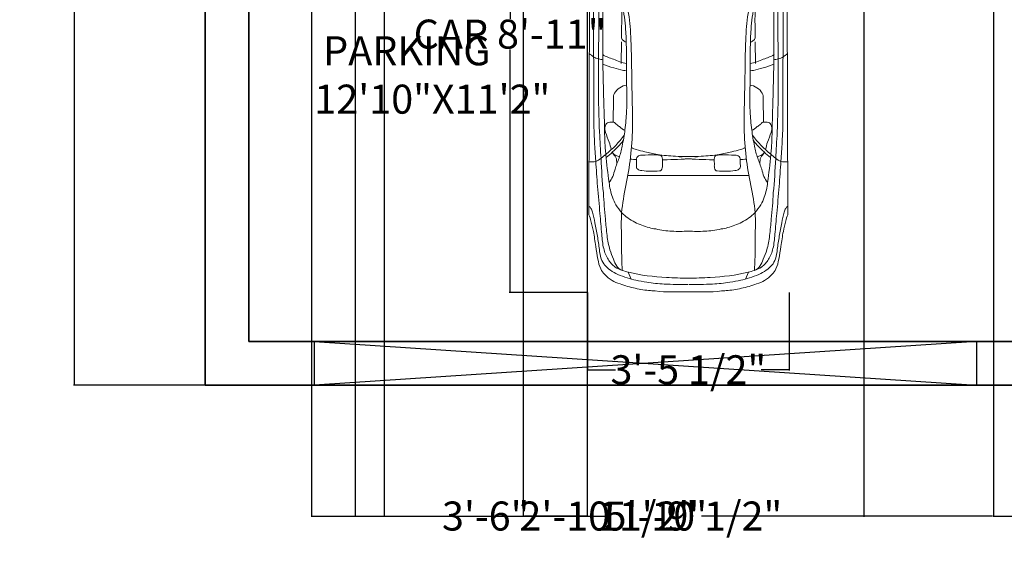
# Model space of a CAD drawing. Units: inches. Extents: x 3398 to 3816, y 15195 to 15771.
# Tile 1 of 10: x 3405 to 3608, y 15195 to 15306. Entities that reach past the tile are written whole.
import ezdxf

# ---------------------------------------------------------------- set-up
doc = ezdxf.new("R2010")
doc.units = ezdxf.units.IN
doc.header["$MEASUREMENT"] = 0
for name, color, linetype, lineweight in [('A-ANNO-DIMS', 2, 'Continuous', 18), ('A-AREA-IDEN', 7, 'Continuous', 25), ('C-PKNG-VEHI', 8, 'Continuous', 13), ('C-PROP', 7, 'Continuous', 35), ('C-SITE-GATE', 4, 'Continuous', 25)]:
    doc.layers.add(name, color=color, linetype=linetype, lineweight=lineweight)
doc.styles.get("Standard").update_dxf_attribs({"font": 'arial.ttf'})
doc.dimstyles.get("Standard").update_dxf_attribs({"dimtxt": 6, "dimasz": 0.18, "dimexe": 0.18, "dimexo": 0.0625, "dimgap": 0.09, "dimtad": 0, "dimtih": 1, "dimtoh": 1, "dimdec": 1, "dimzin": 0, "dimdsep": 46, "dimlunit": 3, "dimtxsty": 'Standard', "dimcen": 0.09, "dimadec": 0, "dimazin": 0, "dimtfac": 1, "dimtdec": 1, "dimtofl": 0, "dimtmove": 0, "dimatfit": 3, "dimfxl": 1, "dimtolj": 1, "dimtzin": 0, "dimarcsym": 0})

# ---------------------------------------------------------------- blocks, each defined once
blk = doc.blocks.new('A$C242571DA')
for p, q in [((1659.9, 1632), (1714.3, 1732.5)), ((1714.3, 1732.5), (3817.1, 1739.9)), ((1638.3, 1618.5), (1625.1, 1632)), ((1625.1, 1632), (1659.9, 1632)), ((1681.8, 1651.6), (2695.2, 1655.3)), ((1699.9, 1699.4), (2984.7, 1695.8)), ((1317.4, 1579.7), (1909.8, 1424.9)), ((1638.3, 1618.5), (2503.3, 1618.5)), ((1659.9, 1548.1), (1638.3, 1618.5)), ((2503.3, 1618.5), (2861.6, 1607.5)), ((1644, 1489.1), (1610.4, 1020.2)), ((2311.9, 1454.3), (2500.6, 1456.9)), ((3007.2, 1526.5), (2808.1, 1525.2)), ((3474.6, 1401.1), (3474.6, 843)), ((4315.2, 1398), (4377.3, 1370.5)), ((1626.1, 1006.5), (1632.8, 719.7)), ((3474.6, 345.6), (3474.6, 903.8)), ((1740.2, 584.9), (1649.3, 586.9)), ((1746.1, 420.6), (1649.3, 420.6)), ((4315.2, 348.7), (4377.3, 376.3)), ((1317.4, 167), (1909.8, 321.9)), ((2311.9, 292.5), (2500.6, 289.8)), ((1659.9, 198.7), (1638.3, 128.2)), ((3007.2, 220.3), (2808.1, 221.6)), ((1638.3, 128.2), (1625.1, 114.7)), ((1625.1, 114.7), (1659.9, 114.7)), ((1638.3, 128.2), (2503.3, 128.2)), ((1659.9, 114.7), (1714.3, 14.2)), ((1681.8, 95.1), (2695.2, 91.4)), ((2503.3, 128.2), (2861.6, 139.2)), ((1699.9, 47.3), (2984.7, 51)), ((1714.3, 14.2), (3817.1, 6.9))]:
    blk.add_line(p, q)
for centre in [(1546.4, 1462.5), (1546.4, 284.2)]:
    blk.add_ellipse(centre, major_axis=(0, 42.9), ratio=0.983266, start_param=4.712389, end_param=10.995574)
for points, knots in [([(0, 873.4), (0, 927.8), (15.6, 1088.6), (25.5, 1309.8), (120.7, 1476.4), (189.2, 1569), (273.5, 1623.1), (369.9, 1666.3), (483, 1694.7), (561.3, 1714.9), (604.6, 1715.7)], [0, 0, 0, 0, 0.16039, 0.479033, 0.632967, 0.722015, 0.817474, 0.927562, 1.03733, 1.167094, 1.167094, 1.167094, 1.167094]), ([(604.6, 1715.7), (545.5, 1714.5), (448.5, 1664.6), (320.8, 1610.6), (225.4, 1521.2), (147.3, 1390.5), (121.7, 1275.2), (113.6, 1208.7)], [0, 0, 0, 0, 0.1772572, 0.3124951, 0.4151678, 0.5597243, 0.7575412, 0.7575412, 0.7575412, 0.7575412]), ([(722.7, 1726.6), (720.8, 1714.9), (694.5, 1689.9), (643, 1671.8), (573.6, 1655.4), (508.5, 1647), (455.2, 1634.7), (428.7, 1627.3), (416.9, 1624.1)], [0, 0, 0, 0, 0.034703, 0.0959761, 0.1659336, 0.2471559, 0.2929944, 0.3295918, 0.3295918, 0.3295918, 0.3295918]), ([(604.6, 1715.7), (642.1, 1723.4), (788.5, 1729.2), (1039.3, 1732.2), (1344.5, 1729.9), (1542, 1733.1), (1633.8, 1733.7)], [0, 0, 0, 0, 0.114897, 0.437061, 0.754269, 1.029686, 1.029686, 1.029686, 1.029686]), ([(1043.6, 1729.2), (1048.6, 1717.9), (1080.9, 1704.2), (1138.6, 1687.6), (1237.7, 1685.6), (1394.7, 1691.3), (1521.7, 1692.4), (1601.5, 1692.7)], [0, 0, 0, 0, 0.0364992, 0.0923739, 0.1867837, 0.3273982, 0.5667068, 0.5667068, 0.5667068, 0.5667068]), ([(1356.8, 1732.2), (1357.1, 1712.8), (1360, 1678.8), (1363.9, 1630.5), (1383.3, 1613.5), (1391, 1607.2)], [0, 0, 0, 0, 1.462159, 2.651105, 3.386321, 3.386321, 3.386321, 3.386321]), ([(1714.3, 1732.5), (1707.7, 1737.6), (1683.3, 1753), (1628.7, 1741.2), (1605.6, 1691.5), (1561.7, 1652.4), (1594.1, 1610.3), (1627.9, 1608.3), (1638.3, 1618.5)], [0, 0, 0, 0, 0.024864, 0.0846267, 0.1362471, 0.1900683, 0.2245199, 0.2681841, 0.2681841, 0.2681841, 0.2681841]), ([(2414.7, 1735), (2424.9, 1723.3), (2447.2, 1698.8), (2461.2, 1657.6), (2468.1, 1629), (2468, 1616.1)], [1.808086, 1.808086, 1.808086, 1.808086, 2.918874, 4.131288, 5.10151, 5.10151, 5.10151, 5.10151]), ([(3356.5, 1739.4), (3354.9, 1719.2), (3360.8, 1678.2), (3324, 1631.5), (3255.4, 1544.3), (3187.1, 1476.2), (3125.2, 1432.2)], [0, 0, 0, 0, 0.0597371, 0.1139981, 0.1672498, 0.3938869, 0.3938869, 0.3938869, 0.3938869]), ([(3745.3, 1736.8), (3748.5, 1730.1), (3764.2, 1717.1), (3811.5, 1698.6), (3894.7, 1686.7), (4002.9, 1663.2), (4107.9, 1648.7), (4195.8, 1638.3), (4258.6, 1603.2), (4302.1, 1549.7), (4339.9, 1483.8), (4365.2, 1407.6), (4389.6, 1324.4), (4397.9, 1266.9), (4401.8, 1235.2)], [0, 0, 0, 0, 0.0219205, 0.0572122, 0.1522539, 0.2718866, 0.3894011, 0.4710097, 0.5346344, 0.5986698, 0.6733118, 0.758696, 0.8351341, 0.9293726, 0.9293726, 0.9293726, 0.9293726]), ([(3817.1, 1739.9), (3833.2, 1729.7), (3882.9, 1718.2), (3973.3, 1695.2), (4085.1, 1680.5), (4193.8, 1662.8), (4280.6, 1644.3), (4343.9, 1598.1), (4390, 1540.3), (4427.4, 1448.7), (4457.8, 1336.6), (4475.7, 1233.4), (4478.4, 1175.1), (4479.3, 1161.6)], [0, 0, 0, 0, 0.056668, 0.14946, 0.28161, 0.392935, 0.481686, 0.542967, 0.622845, 0.69797, 0.833643, 0.965665, 1.00577, 1.00577, 1.00577, 1.00577]), ([(310.7, 1637.3), (282.5, 1613.7), (230.1, 1569.9), (148.7, 1486.2), (84.8, 1361.3), (60, 1219), (32.6, 1054.3), (25.1, 944.9), (25.1, 873.4)], [0, 0, 0, 0, 0.1095129, 0.2035347, 0.3452507, 0.5161382, 0.6275464, 0.8383798, 0.8383798, 0.8383798, 0.8383798]), ([(426.8, 1656.7), (428.5, 1646.6), (426.9, 1625), (399.8, 1616.6), (368.1, 1593.9), (328, 1564.6), (271.6, 1523.9), (237, 1451.9), (196.2, 1376.7), (183.8, 1314.9), (170, 1279.6), (157.2, 1254.2), (133.3, 1244.4), (118.6, 1242.9)], [0, 0, 0, 0, 0.0304541, 0.0502818, 0.0786089, 0.1479133, 0.1986294, 0.2831705, 0.3780326, 0.4523267, 0.4667809, 0.4902599, 0.5347198, 0.5347198, 0.5347198, 0.5347198]), ([(323.7, 1557.5), (344.8, 1571.9), (400.4, 1585.1), (516, 1606.8), (680.3, 1625.8), (885.4, 1635.7), (1116.8, 1642.2), (1346.1, 1644.2), (1504.7, 1644.7), (1574, 1645.7)], [0, 0, 0, 0, 0.076148, 0.165903, 0.355672, 0.569871, 0.782325, 1.050047, 1.257936, 1.257936, 1.257936, 1.257936]), ([(1574, 1645.7), (1572.9, 1638), (1574.1, 1622), (1559.9, 1618.7), (1555.2, 1617.8)], [0, 0, 0, 0, 0.02274132, 0.03717479, 0.03717479, 0.03717479, 0.03717479]), ([(2695.2, 1655.3), (2829.9, 1655.3), (3041.2, 1651.4), (3351.3, 1630.7), (3527.5, 1623.2), (3626.6, 1612)], [0, 0, 0, 0, 0.4042759, 0.6333827, 0.9326252, 0.9326252, 0.9326252, 0.9326252]), ([(2984.7, 1695.8), (3051, 1695.6), (3172.1, 1691.3), (3367.4, 1677.6), (3575.2, 1664.3), (3788.2, 1643.6), (3968, 1628.1), (4103.8, 1616.8), (4203.6, 1578.1), (4271.8, 1519.5), (4300.6, 1452.1), (4341.7, 1305.3), (4361.8, 1111.2), (4367.5, 936.8), (4367.5, 873.4)], [0, 0, 0, 0, 0.198873, 0.363323, 0.587433, 0.823543, 1.004622, 1.129816, 1.230113, 1.320655, 1.388577, 1.443334, 1.771447, 1.958652, 1.958652, 1.958652, 1.958652]), ([(1317.4, 1579.7), (1227.8, 1586.1), (1036, 1584.8), (741.2, 1572.5), (486.1, 1553.3), (333.3, 1534.3), (283.3, 1528.5)], [0, 0, 0, 0, 0.269375, 0.574535, 0.885339, 1.036319, 1.036319, 1.036319, 1.036319]), ([(1555.2, 1617.8), (1527.7, 1617.8), (1472.5, 1620.4), (1392.7, 1608.8), (1318.5, 1591), (1249.4, 1545.5), (1201.4, 1466.7), (1142.8, 1385.7), (1104.8, 1240.4), (1076, 1072.3), (1056.4, 932.4), (1056.4, 873.4)], [0, 0, 0, 0, 0.082256, 0.165174, 0.241383, 0.30939, 0.405348, 0.511507, 0.603349, 0.843635, 1.017671, 1.017671, 1.017671, 1.017671]), ([(1317.4, 1579.7), (1296.6, 1555.5), (1247.9, 1494.4), (1177.6, 1350.5), (1124.2, 1137.4), (1105.5, 964.9), (1105.5, 873.4)], [0, 0, 0, 0, 0.0947759, 0.2311242, 0.4700259, 0.7400315, 0.7400315, 0.7400315, 0.7400315]), ([(1372.8, 1563.1), (1357.2, 1545), (1321.6, 1490.1), (1277, 1385.7), (1232.8, 1244.2), (1211.1, 1069.4), (1196.8, 942.4), (1196.8, 873.4)], [0, 0, 0, 0, 0.0708922, 0.1925846, 0.3348457, 0.5072814, 0.7109928, 0.7109928, 0.7109928, 0.7109928]), ([(3535.9, 1563.1), (3520.1, 1550.9), (3484.4, 1526.1), (3408.2, 1510.9), (3323.4, 1473.1), (3207.9, 1445), (3072.6, 1422.2), (2866.9, 1404.6), (2626.4, 1412.9), (2396.7, 1410.8), (2200.9, 1416.9), (2001.3, 1438.2), (1732.1, 1525.9), (1527.9, 1578.9), (1407.5, 1610.7)], [0, 0, 0, 0, 0.05975, 0.126928, 0.230034, 0.336675, 0.482225, 0.641324, 0.954906, 1.203173, 1.330375, 1.542773, 1.802261, 2.175545, 2.175545, 2.175545, 2.175545]), ([(2424, 1618.7), (2441.5, 1589.9), (2464.2, 1518.9), (2495.4, 1450.9), (2501.6, 1411.3)], [0, 0, 0, 0, 0.1000351, 0.2184418, 0.2184418, 0.2184418, 0.2184418]), ([(2507.7, 1618.4), (2521, 1587.7), (2536.6, 1527.1), (2559.6, 1458.5), (2563.3, 1420.6), (2563.8, 1411.4)], [0, 0, 0, 0, 2.528586, 4.711885, 5.408215, 5.408215, 5.408215, 5.408215]), ([(2861.6, 1607.5), (2921.1, 1607.3), (3047.2, 1600.8), (3191.4, 1602), (3356.6, 1584.1), (3498.3, 1570.6), (3623.2, 1549.4), (3664.1, 1533.3)], [0, 0, 0, 0, 0.1783018, 0.3787173, 0.431954, 0.6762374, 0.8077184, 0.8077184, 0.8077184, 0.8077184]), ([(3248.1, 1545.2), (3226.9, 1550.4), (3176.1, 1562.1), (3113.7, 1592.9), (3052.6, 1605.3), (3010.4, 1578.8), (3010.3, 1545.3), (3010.3, 1515.9), (3033.7, 1500.1), (3052.6, 1465.2), (3078.9, 1443.5), (3084, 1424.4)], [0, 0, 0, 0, 0.0655106, 0.1550445, 0.2094604, 0.2438604, 0.287164, 0.3001388, 0.3275984, 0.3616951, 0.4200969, 0.4200969, 0.4200969, 0.4200969]), ([(3319, 1587.1), (3303.3, 1568.1), (3256.9, 1516.7), (3206.7, 1467.3), (3171.4, 1439.5)], [0, 0, 0, 0, 1.868162, 5.271297, 5.271297, 5.271297, 5.271297]), ([(3626.6, 1612), (3702.5, 1609.1), (3826.2, 1596.8), (3991.4, 1583.2), (4111.7, 1562.4), (4212.2, 1522.7), (4290.4, 1488), (4300.7, 1447.5)], [0, 0, 0, 0, 0.2277977, 0.3719478, 0.4996814, 0.5863441, 0.709615, 0.709615, 0.709615, 0.709615]), ([(1909.8, 1424.9), (1933.5, 1418.7), (1995.6, 1407.6), (2094.4, 1385.8), (2211.8, 1377.1), (2419, 1366.9), (2704.7, 1366.5), (3032.7, 1354.2), (3316.2, 1371), (3558.7, 1415.9), (3789.1, 1461.7), (4028.9, 1452.9), (4196.2, 1455.2), (4292.7, 1447.9), (4300.7, 1447.5)], [0, 0, 0, 0, 0.073325, 0.188896, 0.303039, 0.425821, 0.811242, 1.159737, 1.41058, 1.660623, 1.899627, 2.11145, 2.377727, 2.401703, 2.401703, 2.401703, 2.401703]), ([(1997.2, 1450.5), (2039.7, 1454.5), (2126.7, 1451.9), (2219.8, 1454.5), (2287.1, 1456.9), (2305.7, 1434.4), (2313.2, 1419.9), (2315.8, 1413.5)], [0, 0, 0, 0, 3.267856, 6.568708, 7.399663, 8.099385, 8.621705, 8.621705, 8.621705, 8.621705]), ([(2808.1, 1525.2), (2791.9, 1525.1), (2751.9, 1519.7), (2710.6, 1472.6), (2690, 1431.1), (2690.5, 1409.6)], [0, 0, 0, 0, 0.0486628, 0.1144515, 0.1777721, 0.1777721, 0.1777721, 0.1777721]), ([(3275.5, 1532.8), (3287.5, 1528.3), (3299.8, 1504.9), (3308.4, 1482.5), (3311.7, 1472.6)], [0, 0, 0, 0, 0.983949, 1.771691, 1.771691, 1.771691, 1.771691]), ([(3372.2, 1495.3), (3354.4, 1496.8), (3316, 1494.7), (3291.6, 1525.8), (3275.5, 1532.8)], [0, 0, 0, 0, 0.0535488, 0.1060573, 0.1060573, 0.1060573, 0.1060573]), ([(3664.1, 1533.3), (3687, 1526), (3734.8, 1502.3), (3816.7, 1444.8), (3884.1, 1342.9), (3925.1, 1239.9), (3937.3, 1177), (3940.4, 1157.6)], [0, 0, 0, 0, 0.0720749, 0.1581284, 0.2958089, 0.4262456, 0.4842292, 0.4842292, 0.4842292, 0.4842292]), ([(113.6, 1208.7), (215.2, 1238.6), (443.2, 1284.9), (788, 1338.7), (1029.5, 1370.7), (1146.4, 1378.6)], [0, 0, 0, 0, 0.317374, 0.69576, 1.04714, 1.04714, 1.04714, 1.04714]), ([(1898.5, 1426.2), (1889, 1420.6), (1871, 1397.2), (1856.4, 1345.2), (1867.7, 1233.5), (1864.3, 1132.3), (1863, 1038.5), (1876.9, 1022.3), (1884.5, 1015.7)], [0, 0, 0, 0, 0.842998, 2.122875, 3.997599, 9.174838, 10.012722, 10.751336, 10.751336, 10.751336, 10.751336]), ([(1969.6, 1407.3), (1960.5, 1369.8), (1927, 1259.1), (1890.9, 1078.4), (1874.3, 933), (1874.3, 864.4)], [0, 0, 0, 0, 0.1139079, 0.3411539, 0.543502, 0.543502, 0.543502, 0.543502]), ([(3231.5, 1368.3), (3240.8, 1356.2), (3253.1, 1315.7), (3271.9, 1240.7), (3297.9, 1127.9), (3310.5, 974.6), (3311.2, 858.3), (3311.6, 794.4)], [0, 0, 0, 0, 0.0451009, 0.1211996, 0.2308505, 0.385263, 0.5739042, 0.5739042, 0.5739042, 0.5739042]), ([(3294.8, 1174.5), (3294.8, 1207.4), (3299.6, 1249.5), (3298.3, 1303.9), (3326.3, 1329), (3363.9, 1320.7), (3399.3, 1329.3), (3422.1, 1315.7), (3430.7, 1297.9), (3438.7, 1234.2), (3439.6, 1174.4), (3434.7, 1112.2), (3418.9, 1102), (3395.9, 1098.6), (3362.6, 1100.9), (3331.1, 1096.6), (3298.8, 1107.6), (3297.3, 1140.3), (3294.8, 1160.9), (3294.8, 1174.5)], [0, 0, 0, 0, 0.0969044, 0.1295913, 0.1506192, 0.1985921, 0.2360698, 0.2557908, 0.2719711, 0.2929882, 0.44406, 0.4519132, 0.4720918, 0.4918599, 0.5228758, 0.5707096, 0.5892096, 0.6145759, 0.654681, 0.654681, 0.654681, 0.654681]), ([(113.6, 1208.7), (103.3, 1207), (83.6, 1187.6), (76.5, 1122.2), (68.2, 1017.3), (53.4, 925), (53.4, 873.4)], [0, 0, 0, 0, 0.0314754, 0.0702057, 0.1915753, 0.3439346, 0.3439346, 0.3439346, 0.3439346]), ([(135.5, 1213.1), (139.1, 1211.8), (138.4, 1193.3), (132.6, 1168.3), (118.8, 1111.9), (115.6, 1058.9), (109, 974.6), (102.4, 920.1), (102.4, 873.4)], [0, 0, 0, 0, 0.0114788, 0.0403472, 0.0875838, 0.1755608, 0.1991501, 0.3369659, 0.3369659, 0.3369659, 0.3369659]), ([(4401.8, 1235.2), (4411.9, 1185.3), (4421.6, 1065.8), (4424.1, 946.5), (4424.1, 878)], [0, 0, 0, 0, 0.1502861, 0.3522699, 0.3522699, 0.3522699, 0.3522699]), ([(3940.4, 1157.6), (3949.9, 1111), (3964.3, 1016.4), (3960.5, 921), (3959.8, 873.4)], [0, 0, 0, 0, 0.140379, 0.2808468, 0.2808468, 0.2808468, 0.2808468]), ([(1311.3, 873.4), (1311.2, 902.4), (1309.2, 950.9), (1315, 1002.2), (1314.2, 1039.4), (1332.1, 1044.9), (1345.7, 1044.2), (1356.8, 1028.5), (1359.2, 970.2), (1361.5, 917.6), (1362.9, 873.4)], [0, 0, 0, 0, 0.0857277, 0.1381048, 0.1641986, 0.1769751, 0.1890325, 0.2028129, 0.2286049, 0.3592554, 0.3592554, 0.3592554, 0.3592554]), ([(3339.2, 1099), (3339.1, 1094.8), (3336.4, 1010.6), (3333.2, 926.3), (3330, 846.2)], [11.235438, 11.235438, 11.235438, 11.235438, 11.552536, 17.586883, 17.586883, 17.586883, 17.586883]), ([(1626.1, 1006.5), (1623.5, 1013), (1603.1, 1029.4), (1559.1, 995), (1523, 951.9), (1480.3, 878.3), (1430.5, 774.3), (1385.5, 658.5), (1343.7, 551.3), (1343, 461.7), (1380.3, 386.9), (1428.2, 329.9), (1480.1, 294.6), (1509.8, 257.4), (1524.8, 232.6), (1528, 222.1)], [0, 0, 0, 0, 0.527288, 1.647451, 3.487558, 5.099073, 7.968657, 12.238313, 14.475187, 16.613757, 18.744202, 20.639343, 22.223389, 23.452731, 24.286529, 24.286529, 24.286529, 24.286529]), ([(3231.5, 378.5), (3240.8, 390.5), (3253.1, 431), (3271.9, 506.1), (3297.9, 618.9), (3310.5, 772.1), (3311.2, 888.4), (3311.6, 952.4)], [0, 0, 0, 0, 0.0451009, 0.1211996, 0.2308505, 0.385263, 0.5739042, 0.5739042, 0.5739042, 0.5739042]), ([(0, 873.4), (0, 819), (15.6, 658.1), (25.5, 437), (120.7, 270.3), (189.2, 177.8), (273.5, 123.7), (369.9, 80.4), (483, 52), (561.3, 31.9), (604.6, 31)], [0, 0, 0, 0, 0.16039, 0.479033, 0.632967, 0.722015, 0.817474, 0.927562, 1.03733, 1.167094, 1.167094, 1.167094, 1.167094]), ([(310.7, 109.5), (282.5, 133.1), (230.1, 176.9), (148.7, 260.5), (84.8, 385.5), (60, 527.8), (32.6, 692.4), (25.1, 801.9), (25.1, 873.4)], [0, 0, 0, 0, 0.1095129, 0.2035347, 0.3452507, 0.5161382, 0.6275464, 0.8383798, 0.8383798, 0.8383798, 0.8383798]), ([(113.6, 538.1), (103.3, 539.8), (83.6, 559.2), (76.5, 624.5), (68.2, 729.4), (53.4, 821.7), (53.4, 873.4)], [0, 0, 0, 0, 0.0314754, 0.0702057, 0.1915753, 0.3439346, 0.3439346, 0.3439346, 0.3439346]), ([(135.5, 533.6), (139.1, 534.9), (138.4, 553.4), (132.6, 578.4), (118.8, 634.9), (115.6, 687.8), (109, 772.2), (102.4, 826.7), (102.4, 873.4)], [0, 0, 0, 0, 0.0114788, 0.0403472, 0.0875838, 0.1755608, 0.1991501, 0.3369659, 0.3369659, 0.3369659, 0.3369659]), ([(1555.2, 129), (1527.7, 129), (1472.5, 126.3), (1392.7, 138), (1318.5, 155.7), (1249.4, 201.3), (1201.4, 280.1), (1142.8, 361.1), (1104.8, 506.4), (1076, 674.5), (1056.4, 814.4), (1056.4, 873.4)], [0, 0, 0, 0, 0.082256, 0.165174, 0.241383, 0.30939, 0.405348, 0.511507, 0.603349, 0.843635, 1.017671, 1.017671, 1.017671, 1.017671]), ([(1317.4, 167), (1296.6, 191.2), (1247.9, 252.4), (1177.6, 396.3), (1124.2, 609.4), (1105.5, 781.8), (1105.5, 873.4)], [0, 0, 0, 0, 0.0947759, 0.2311242, 0.4700259, 0.7400315, 0.7400315, 0.7400315, 0.7400315]), ([(1372.8, 183.6), (1357.2, 201.8), (1321.6, 256.7), (1277, 361), (1232.8, 502.6), (1211.1, 677.3), (1196.8, 804.3), (1196.8, 873.4)], [0, 0, 0, 0, 0.0708922, 0.1925846, 0.3348457, 0.5072814, 0.7109928, 0.7109928, 0.7109928, 0.7109928]), ([(1311.3, 873.4), (1311.2, 844.3), (1309.2, 795.8), (1315, 744.6), (1314.2, 707.4), (1332.1, 701.9), (1345.7, 702.6), (1356.8, 718.2), (1359.2, 776.6), (1361.5, 829.1), (1362.9, 873.4)], [0, 0, 0, 0, 0.0857277, 0.1381048, 0.1641986, 0.1769751, 0.1890325, 0.2028129, 0.2286049, 0.3592554, 0.3592554, 0.3592554, 0.3592554]), ([(1969.6, 339.5), (1960.5, 377), (1926.9, 487.6), (1892.9, 662.7), (1874.3, 801.8), (1874.3, 864.4)], [0, 0, 0, 0, 0.1139079, 0.3411539, 0.5260188, 0.5260188, 0.5260188, 0.5260188]), ([(2984.7, 51), (3051, 51.1), (3172.1, 55.5), (3367.4, 69.2), (3575.2, 82.5), (3788.2, 103.1), (3968, 118.7), (4103.8, 130), (4203.6, 168.6), (4271.8, 227.3), (4300.6, 294.7), (4341.7, 441.5), (4361.8, 635.5), (4367.5, 809.9), (4367.5, 873.4)], [0, 0, 0, 0, 0.198873, 0.363323, 0.587433, 0.823543, 1.004622, 1.129816, 1.230113, 1.320655, 1.388577, 1.443334, 1.771447, 1.958652, 1.958652, 1.958652, 1.958652]), ([(3339.2, 647.8), (3339.1, 652), (3336.4, 736.2), (3333.2, 820.5), (3330, 900.6)], [11.235438, 11.235438, 11.235438, 11.235438, 11.552536, 17.586883, 17.586883, 17.586883, 17.586883]), ([(3940.4, 589.1), (3949.9, 635.7), (3964.3, 730.4), (3960.5, 825.8), (3959.8, 873.4)], [0, 0, 0, 0, 0.140379, 0.2808468, 0.2808468, 0.2808468, 0.2808468]), ([(4401.8, 511.5), (4411.9, 561.5), (4421.6, 681), (4424.1, 800.3), (4424.1, 868.8)], [0, 0, 0, 0, 0.1502861, 0.3522699, 0.3522699, 0.3522699, 0.3522699]), ([(1639.2, 326.1), (1635.3, 323.6), (1629, 318.4), (1613.1, 314.9), (1612, 324.2), (1613.2, 330.4), (1619, 337.5), (1629, 345.7), (1637.9, 366.1), (1649, 404.8), (1656.3, 472.9), (1656.2, 543.1), (1644.6, 610.9), (1623, 651.2), (1615, 684.3), (1598.5, 691.2), (1604, 696.6), (1610.3, 699.7), (1618.8, 698.9), (1625.9, 701.3), (1638.1, 698.6), (1633, 713.4), (1632.8, 719.7)], [0, 0, 0, 0, 0.0138597, 0.0278304, 0.0329137, 0.0379971, 0.0465756, 0.0592704, 0.0762214, 0.1105991, 0.1789801, 0.2766959, 0.3173629, 0.3800771, 0.4110544, 0.4160421, 0.4210284, 0.4277212, 0.4387433, 0.4448131, 0.4508005, 0.4694463, 0.4694463, 0.4694463, 0.4694463]), ([(1740.2, 584.9), (1737.8, 571.7), (1749.5, 644.3), (1766.4, 664.5), (1792.2, 700.2), (1821.5, 709.7), (1853.1, 703.9), (1874, 668.4), (1904.5, 622.6), (1915.6, 557.2), (1915.1, 484.2), (1905.7, 417.6), (1884.9, 362.8), (1859.3, 329.1), (1831.3, 318.1), (1810.8, 322.7), (1792.2, 329.3), (1777.9, 350.3), (1753, 385.9), (1737.9, 465.8), (1728.8, 497.3), (1742.4, 597.6), (1740.2, 584.9)], [0, 0, 0, 0, 0.03969, 0.089634, 0.13125, 0.1542862, 0.1797268, 0.2207266, 0.2680991, 0.3447665, 0.4095645, 0.4843001, 0.541515, 0.5817687, 0.6060665, 0.6262474, 0.6436722, 0.6634686, 0.6988791, 0.7758465, 0.8696394, 0.907731, 0.907731, 0.907731, 0.907731]), ([(1863.4, 685.6), (1863.6, 693.5), (1865.3, 711), (1876.9, 724.5), (1884.5, 731)], [9.436432, 9.436432, 9.436432, 9.436432, 10.012722, 10.751336, 10.751336, 10.751336, 10.751336]), ([(1764.9, 587), (1765.6, 590.8), (1766.4, 595.5), (1768.5, 605.7), (1769.7, 611.3), (1773.4, 626.6), (1775.6, 633), (1779.7, 642.1), (1781.6, 644.9), (1785.7, 650.6), (1787.1, 652.5), (1793, 660.3), (1797.4, 666.2), (1804.2, 673.7), (1806.8, 676.1), (1811.1, 679.4), (1812.9, 680.5), (1816.8, 682.1), (1818.8, 682.7), (1824.4, 683.5), (1828.3, 683.2), (1832.5, 682), (1833.6, 681.5), (1836, 680.2), (1837.9, 678.7), (1842.4, 673.7), (1844.9, 670.1), (1850.3, 661.7), (1853.4, 656.6), (1859.3, 647.3), (1862.1, 642.8), (1868.3, 632.6), (1871.4, 626.9), (1876.7, 615.7), (1878.9, 609.8), (1882.8, 597.4), (1884.4, 590.8), (1888.3, 570.5), (1889.7, 556.1), (1891.2, 527.4), (1891.1, 513.1), (1888.9, 470), (1885.1, 441.2), (1874.3, 404), (1870.6, 393.8), (1863.5, 378.7), (1860.6, 373.4), (1854.4, 363.6), (1851.2, 359.2), (1845, 352.6), (1842, 350.2), (1835.8, 346.4), (1832.6, 345.3), (1828.8, 344.6), (1827.9, 344.6), (1824.6, 344.9), (1822.6, 345.2), (1817.8, 346.4), (1814.9, 347.3), (1810.9, 348.7), (1809.4, 349.4), (1808.3, 350.1), (1808.1, 350.2), (1807.3, 351), (1806.7, 351.6), (1804.7, 354), (1803.1, 356.2), (1799.6, 361.3), (1798, 363.7), (1794.9, 368.2), (1793.4, 370.4), (1789.2, 376.9), (1786.7, 381), (1782.4, 389.3), (1780.5, 393.6), (1776.9, 403), (1775.2, 408), (1770.7, 423.5), (1768.3, 434.2), (1764.9, 450.5), (1763.6, 456.4), (1761.4, 466.8), (1760.4, 471.4), (1758.1, 484.4), (1757.3, 492.6), (1757.5, 510.7), (1757.8, 516.5), (1758.6, 528.4), (1759.1, 534.3), (1761.1, 553.9), (1763.1, 570.6), (1764.4, 581.5), (1764.6, 583), (1764.7, 585), (1764.8, 585.5), (1764.8, 586.5), (1764.8, 586.7), (1764.9, 587)], [0.497033, 0.497033, 0.497033, 0.497033, 0.723444, 0.723444, 0.974636, 0.974636, 1.50964, 1.50964, 2.044645, 2.044645, 2.271061, 2.271061, 2.862376, 2.862376, 3.217654, 3.217654, 3.537253, 3.537253, 3.856852, 3.856852, 4.368613, 4.368613, 4.584627, 4.584627, 4.99269, 4.99269, 5.400753, 5.400753, 5.808816, 5.808816, 6.216879, 6.216879, 6.778716, 6.778716, 7.350371, 7.350371, 7.922025, 7.922025, 9.065335, 9.065335, 10.208644, 10.208644, 12.495263, 12.495263, 13.409896, 13.409896, 13.929088, 13.929088, 14.44828, 14.44828, 14.909885, 14.909885, 15.371489, 15.371489, 15.62524, 15.62524, 15.87899, 15.87899, 16.120875, 16.120875, 16.36276, 16.36276, 16.51635, 16.51635, 16.669941, 16.669941, 16.921521, 16.921521, 17.136676, 17.136676, 17.351831, 17.351831, 17.782142, 17.782142, 18.204974, 18.204974, 18.627807, 18.627807, 19.473473, 19.473473, 19.978923, 19.978923, 20.484372, 20.484372, 21.475119, 21.475119, 21.859144, 21.859144, 22.162884, 22.162884, 22.770362, 22.770362, 22.900493, 22.900493, 22.951221, 22.951221, 22.964298, 22.964298, 22.964298, 22.964298]), ([(1863.7, 379.4), (1862.6, 384.2), (1857.6, 413.7), (1866.5, 501.6), (1865.2, 581.4), (1864.1, 639.5)], [1.749253, 1.749253, 1.749253, 1.749253, 2.122875, 3.997599, 8.307432, 8.307432, 8.307432, 8.307432]), ([(3294.8, 572.3), (3294.8, 539.4), (3299.6, 497.2), (3298.3, 442.9), (3326.3, 417.8), (3363.9, 426), (3399.3, 417.5), (3422.1, 431), (3430.7, 448.9), (3438.7, 512.5), (3439.6, 572.4), (3434.7, 634.6), (3418.9, 644.7), (3395.9, 648.2), (3362.6, 645.9), (3331.1, 650.1), (3298.8, 639.2), (3297.3, 606.5), (3294.8, 585.9), (3294.8, 572.3)], [0, 0, 0, 0, 0.0969044, 0.1295913, 0.1506192, 0.1985921, 0.2360698, 0.2557908, 0.2719711, 0.2929882, 0.44406, 0.4519132, 0.4720918, 0.4918599, 0.5228758, 0.5707096, 0.5892096, 0.6145759, 0.654681, 0.654681, 0.654681, 0.654681]), ([(604.6, 31), (545.5, 32.3), (448.5, 82.2), (320.8, 136.1), (225.4, 225.5), (147.3, 356.2), (121.7, 471.5), (113.6, 538.1)], [0, 0, 0, 0, 0.1772572, 0.3124951, 0.4151678, 0.5597243, 0.7575412, 0.7575412, 0.7575412, 0.7575412]), ([(113.6, 538.1), (215.2, 508.2), (443.2, 461.9), (788, 408.1), (1029.5, 376), (1146.4, 368.2)], [0, 0, 0, 0, 0.317374, 0.69576, 1.04714, 1.04714, 1.04714, 1.04714]), ([(3664.1, 213.5), (3687, 220.8), (3734.8, 244.4), (3816.7, 302), (3884.1, 403.8), (3925.1, 506.9), (3937.3, 569.7), (3940.4, 589.1)], [0, 0, 0, 0, 0.0720749, 0.1581284, 0.2958089, 0.4262456, 0.4842292, 0.4842292, 0.4842292, 0.4842292]), ([(3817.1, 6.9), (3833.2, 17), (3882.9, 28.6), (3973.3, 51.5), (4085.1, 66.3), (4193.8, 84), (4280.6, 102.4), (4343.9, 148.6), (4390, 206.4), (4427.4, 298), (4457.8, 410.1), (4475.7, 513.3), (4478.4, 571.6), (4479.3, 585.2)], [0, 0, 0, 0, 0.056668, 0.14946, 0.28161, 0.392935, 0.481686, 0.542967, 0.622845, 0.69797, 0.833643, 0.965665, 1.00577, 1.00577, 1.00577, 1.00577]), ([(426.8, 90), (428.5, 100.2), (426.9, 121.8), (399.8, 130.1), (368.1, 152.8), (328, 182.2), (271.6, 222.8), (237, 294.9), (196.2, 370.1), (183.8, 431.9), (170, 467.2), (157.2, 492.6), (133.3, 502.4), (118.6, 503.9)], [0, 0, 0, 0, 0.0304541, 0.0502818, 0.0786089, 0.1479133, 0.1986294, 0.2831705, 0.3780326, 0.4523267, 0.4667809, 0.4902599, 0.5347198, 0.5347198, 0.5347198, 0.5347198]), ([(3745.3, 10), (3748.5, 16.7), (3764.2, 29.7), (3811.5, 48.1), (3894.7, 60.1), (4002.9, 83.6), (4107.9, 98), (4195.8, 108.4), (4258.6, 143.5), (4302.1, 197), (4339.9, 262.9), (4365.2, 339.2), (4389.6, 422.4), (4397.9, 479.8), (4401.8, 511.5)], [0, 0, 0, 0, 0.0219205, 0.0572122, 0.1522539, 0.2718866, 0.3894011, 0.4710097, 0.5346344, 0.5986698, 0.6733118, 0.758696, 0.8351341, 0.9293726, 0.9293726, 0.9293726, 0.9293726]), ([(1898.5, 320.6), (1889, 326.2), (1880.8, 336.8), (1874.8, 348.3), (1874, 349.7)], [0, 0, 0, 0, 0.8429982, 0.9626806, 0.9626806, 0.9626806, 0.9626806]), ([(1909.8, 321.9), (1933.5, 328.1), (1995.6, 339.2), (2094.4, 361), (2211.8, 369.6), (2419, 379.8), (2704.7, 380.3), (3032.7, 392.6), (3316.2, 375.8), (3558.7, 330.9), (3789.1, 285.1), (4028.9, 293.9), (4196.2, 291.5), (4292.7, 298.8), (4300.7, 299.2)], [0, 0, 0, 0, 0.073325, 0.188896, 0.303039, 0.425821, 0.811242, 1.159737, 1.41058, 1.660623, 1.899627, 2.11145, 2.377727, 2.401703, 2.401703, 2.401703, 2.401703]), ([(3535.9, 183.7), (3520.1, 195.9), (3484.4, 220.6), (3408.2, 235.8), (3323.4, 273.7), (3207.9, 301.8), (3072.6, 324.6), (2866.9, 342.1), (2626.4, 333.8), (2396.7, 335.9), (2200.9, 329.9), (2001.3, 308.6), (1732.1, 220.8), (1527.9, 167.8), (1407.5, 136)], [0, 0, 0, 0, 0.05975, 0.126928, 0.230034, 0.336675, 0.482225, 0.641324, 0.954906, 1.203173, 1.330375, 1.542773, 1.802261, 2.175545, 2.175545, 2.175545, 2.175545]), ([(1997.2, 296.3), (2039.7, 292.2), (2126.7, 294.9), (2219.8, 292.3), (2287.1, 289.9), (2305.7, 312.3), (2313.2, 326.9), (2315.8, 333.2)], [0, 0, 0, 0, 3.267856, 6.568708, 7.399663, 8.099385, 8.621705, 8.621705, 8.621705, 8.621705]), ([(2424, 128), (2441.5, 156.9), (2464.2, 227.8), (2495.4, 295.8), (2501.6, 335.5)], [0, 0, 0, 0, 0.1000351, 0.2184418, 0.2184418, 0.2184418, 0.2184418]), ([(2507.7, 128.3), (2521, 159.1), (2536.6, 219.7), (2559.6, 288.3), (2563.3, 326.1), (2563.8, 335.3)], [0, 0, 0, 0, 2.528586, 4.711885, 5.408215, 5.408215, 5.408215, 5.408215]), ([(2808.1, 221.6), (2791.9, 221.6), (2751.9, 227.1), (2710.6, 274.2), (2690, 315.7), (2690.5, 337.1)], [0, 0, 0, 0, 0.0486628, 0.1144515, 0.1777721, 0.1777721, 0.1777721, 0.1777721]), ([(3248.1, 201.6), (3226.9, 196.3), (3176.1, 184.7), (3113.7, 153.8), (3052.6, 141.4), (3010.4, 168), (3010.3, 201.5), (3010.3, 230.9), (3033.7, 246.6), (3052.6, 281.6), (3078.9, 303.2), (3084, 322.4)], [0, 0, 0, 0, 0.0655106, 0.1550445, 0.2094604, 0.2438604, 0.287164, 0.3001388, 0.3275984, 0.3616951, 0.4200969, 0.4200969, 0.4200969, 0.4200969]), ([(3356.5, 7.4), (3354.9, 27.5), (3360.8, 68.5), (3324, 115.2), (3255.4, 202.5), (3187.1, 270.5), (3125.2, 314.6)], [0, 0, 0, 0, 0.0597371, 0.1139981, 0.1672498, 0.3938869, 0.3938869, 0.3938869, 0.3938869]), ([(3319, 159.7), (3303.3, 178.6), (3256.9, 230), (3206.7, 279.5), (3171.4, 307.2)], [0, 0, 0, 0, 1.868162, 5.271297, 5.271297, 5.271297, 5.271297]), ([(3275.5, 214), (3287.5, 218.5), (3299.8, 241.9), (3308.4, 264.3), (3311.7, 274.2)], [0, 0, 0, 0, 0.983949, 1.771691, 1.771691, 1.771691, 1.771691]), ([(3626.6, 134.7), (3702.5, 137.7), (3826.2, 149.9), (3991.4, 163.5), (4111.7, 184.4), (4212.2, 224.1), (4290.4, 258.8), (4300.7, 299.2)], [0, 0, 0, 0, 0.2277977, 0.3719478, 0.4996814, 0.5863441, 0.709615, 0.709615, 0.709615, 0.709615]), ([(1317.4, 167), (1227.8, 160.7), (1036, 161.9), (741.2, 174.2), (486.1, 193.4), (333.3, 212.5), (283.3, 218.3)], [0, 0, 0, 0, 0.269375, 0.574535, 0.885339, 1.036319, 1.036319, 1.036319, 1.036319]), ([(323.7, 189.2), (344.8, 174.9), (400.4, 161.7), (516, 139.9), (680.3, 121), (885.4, 111), (1116.8, 104.5), (1346.1, 102.5), (1504.7, 102), (1574, 101.1)], [0, 0, 0, 0, 0.076148, 0.165903, 0.355672, 0.569871, 0.782325, 1.050047, 1.257936, 1.257936, 1.257936, 1.257936]), ([(2861.6, 139.2), (2921.1, 139.4), (3047.2, 146), (3191.4, 144.8), (3356.6, 162.6), (3498.3, 176.1), (3623.2, 197.4), (3664.1, 213.5)], [0, 0, 0, 0, 0.1783018, 0.3787173, 0.431954, 0.6762374, 0.8077184, 0.8077184, 0.8077184, 0.8077184]), ([(3372.2, 251.5), (3354.4, 249.9), (3316, 252), (3291.6, 220.9), (3275.5, 214)], [0, 0, 0, 0, 0.0535488, 0.1060573, 0.1060573, 0.1060573, 0.1060573]), ([(722.7, 20.2), (720.8, 31.8), (694.5, 56.8), (643, 75), (573.6, 91.4), (508.5, 99.8), (455.2, 112.1), (428.7, 119.5), (416.9, 122.6)], [0, 0, 0, 0, 0.034703, 0.0959761, 0.1659336, 0.2471559, 0.2929944, 0.3295918, 0.3295918, 0.3295918, 0.3295918]), ([(1356.8, 14.5), (1357.1, 33.9), (1360, 68), (1363.9, 116.3), (1383.3, 133.2), (1391, 139.5)], [0, 0, 0, 0, 1.462159, 2.651105, 3.386321, 3.386321, 3.386321, 3.386321]), ([(1574, 101.1), (1572.9, 108.7), (1574.1, 124.8), (1559.9, 128), (1555.2, 129)], [0, 0, 0, 0, 0.02274132, 0.03717479, 0.03717479, 0.03717479, 0.03717479]), ([(1714.3, 14.2), (1707.7, 9.2), (1683.3, -6.3), (1628.7, 5.5), (1605.6, 55.3), (1561.7, 94.4), (1594.1, 136.5), (1627.9, 138.5), (1638.3, 128.2)], [0, 0, 0, 0, 0.024864, 0.0846267, 0.1362471, 0.1900683, 0.2245199, 0.2681841, 0.2681841, 0.2681841, 0.2681841]), ([(2414.7, 11.8), (2424.9, 23.5), (2447.2, 48), (2461.2, 89.1), (2468.1, 117.8), (2468, 130.7)], [1.808086, 1.808086, 1.808086, 1.808086, 2.918874, 4.131288, 5.10151, 5.10151, 5.10151, 5.10151]), ([(2695.2, 91.4), (2829.9, 91.5), (3041.2, 95.4), (3351.3, 116.1), (3527.5, 123.5), (3626.6, 134.7)], [0, 0, 0, 0, 0.4042759, 0.6333827, 0.9326252, 0.9326252, 0.9326252, 0.9326252]), ([(604.6, 31), (642.1, 23.4), (788.5, 17.5), (1039.3, 14.6), (1344.5, 16.8), (1542, 13.6), (1633.8, 13.1)], [0, 0, 0, 0, 0.114897, 0.437061, 0.754269, 1.029686, 1.029686, 1.029686, 1.029686]), ([(1043.6, 17.6), (1048.6, 28.9), (1080.9, 42.6), (1138.6, 59.2), (1237.7, 61.2), (1394.7, 55.4), (1521.7, 54.3), (1601.5, 54.1)], [0, 0, 0, 0, 0.0364992, 0.0923739, 0.1867837, 0.3273982, 0.5667068, 0.5667068, 0.5667068, 0.5667068])]:
    blk.add_open_spline(points, degree=3, knots=knots)
for points in [[(283.3, 1528.5), (267.8, 1524.6), (251.4, 1527.5), (235.4, 1528.5)], [(3331.9, 1378.1), (3334.2, 1360.4), (3335.9, 1342.5), (3337.3, 1324.5)], [(4479.3, 1161.6), (4491, 1066.2), (4488, 969.5), (4488, 873.4)], [(4479.3, 585.2), (4491, 680.6), (4488, 777.3), (4488, 873.4)], [(3331.9, 368.6), (3334.2, 386.4), (3335.9, 404.3), (3337.3, 422.2)], [(1646.2, 253.1), (1647.8, 277.5), (1640, 301.6), (1639.2, 326.1)], [(283.3, 218.3), (267.8, 222.1), (251.4, 219.2), (235.4, 218.3)]]:
    blk.add_open_spline(points, degree=3)
blk = doc.blocks.new('*D34')
at = {"layer": 'A-ANNO-DIMS', "color": 0, "lineweight": -2, "transparency": 16777216}
for p, q in [((3522.18, 15356.47), (3506.05, 15356.47)), ((3506.23, 15356.29), (3506.23, 15306.28)), ((3506.23, 15249.89), (3506.23, 15299.9)), ((3522.18, 15249.71), (3506.05, 15249.71))]:
    blk.add_line(p, q, dxfattribs=at)
at = {"layer": 'A-ANNO-DIMS', "color": 0, "transparency": 16777216}
for points in [[(3506.2, 15356.29), (3506.26, 15356.29), (3506.23, 15356.47)], [(3506.2, 15249.89), (3506.26, 15249.89), (3506.23, 15249.71)]]:
    blk.add_solid(points, dxfattribs=at)
at = {"layer": 'Defpoints', "color": 0, "transparency": 16777216}
for p in [(3522.24, 15356.47), (3506.23, 15249.71), (3522.24, 15249.71)]:
    blk.add_point(p, dxfattribs=at)
at = {"layer": 'A-ANNO-DIMS', "color": 0, "transparency": 16777216, "insert": (3506.23, 15303.09), "char_height": 6, "attachment_point": 5}
blk.add_mtext('\\A1;CAR 8\'-11"', dxfattribs=at)
blk = doc.blocks.new('*D35')
at = {"layer": 'A-ANNO-DIMS', "color": 0, "lineweight": -2, "transparency": 16777216}
for p, q in [((3522.24, 15249.65), (3522.24, 15233.52)), ((3563.96, 15249.65), (3563.96, 15233.52)), ((3522.42, 15233.7), (3528.04, 15233.7)), ((3563.78, 15233.7), (3558.15, 15233.7))]:
    blk.add_line(p, q, dxfattribs=at)
at = {"layer": 'A-ANNO-DIMS', "color": 0, "transparency": 16777216}
for points in [[(3522.42, 15233.73), (3522.42, 15233.67), (3522.24, 15233.7)], [(3563.78, 15233.73), (3563.78, 15233.67), (3563.96, 15233.7)]]:
    blk.add_solid(points, dxfattribs=at)
at = {"layer": 'Defpoints', "color": 0, "transparency": 16777216}
for p in [(3522.24, 15249.71), (3563.96, 15249.71), (3563.96, 15233.7)]:
    blk.add_point(p, dxfattribs=at)
at = {"layer": 'A-ANNO-DIMS', "color": 0, "transparency": 16777216, "insert": (3543.1, 15233.7), "char_height": 6, "attachment_point": 5}
blk.add_mtext('\\A1;3\'-5 1/2"', dxfattribs=at)
blk = doc.blocks.new('*D38')
at = {"layer": 'A-ANNO-DIMS', "color": 0, "lineweight": -2, "transparency": 16777216}
for p, q in [((3465.13, 15730.52), (3415.96, 15730.52)), ((3416.14, 15730.34), (3416.14, 15483.67)), ((3416.14, 15230.7), (3416.14, 15477.37)), ((3465.74, 15230.52), (3415.96, 15230.52))]:
    blk.add_line(p, q, dxfattribs=at)
at = {"layer": 'A-ANNO-DIMS', "color": 0, "transparency": 16777216}
for points in [[(3416.11, 15730.34), (3416.17, 15730.34), (3416.14, 15730.52)], [(3416.11, 15230.7), (3416.17, 15230.7), (3416.14, 15230.52)]]:
    blk.add_solid(points, dxfattribs=at)
at = {"layer": 'Defpoints', "color": 0, "transparency": 16777216}
for p in [(3416.14, 15730.52), (3465.19, 15730.52), (3465.8, 15230.52)]:
    blk.add_point(p, dxfattribs=at)
at = {"layer": 'A-ANNO-DIMS', "color": 0, "transparency": 16777216, "insert": (3416.14, 15480.52), "char_height": 6, "attachment_point": 5}
blk.add_mtext('\\A1;41\'-8"', dxfattribs=at)
blk = doc.blocks.new('*D39')
at = {"layer": 'A-ANNO-DIMS', "color": 0, "lineweight": -2, "transparency": 16777216}
for p, q in [((3465.19, 15373.46), (3465.19, 15203.29)), ((3606.19, 15373.46), (3606.19, 15203.29)), ((3465.37, 15203.47), (3525.58, 15203.47)), ((3606.01, 15203.47), (3545.8, 15203.47))]:
    blk.add_line(p, q, dxfattribs=at)
at = {"layer": 'A-ANNO-DIMS', "color": 0, "transparency": 16777216}
for points in [[(3465.37, 15203.5), (3465.37, 15203.44), (3465.19, 15203.47)], [(3606.01, 15203.5), (3606.01, 15203.44), (3606.19, 15203.47)]]:
    blk.add_solid(points, dxfattribs=at)
at = {"layer": 'Defpoints', "color": 0, "transparency": 16777216}
for p in [(3465.19, 15373.52), (3606.19, 15373.52), (3606.19, 15203.47)]:
    blk.add_point(p, dxfattribs=at)
at = {"layer": 'A-ANNO-DIMS', "color": 0, "transparency": 16777216, "insert": (3535.69, 15203.47), "char_height": 6, "attachment_point": 5}
blk.add_mtext('\\A1;11\'-9"', dxfattribs=at)
blk = doc.blocks.new('*D41')
at = {"layer": 'A-ANNO-DIMS', "color": 0, "lineweight": -2, "transparency": 16777216}
for p, q in [((3480.19, 15373.46), (3480.19, 15203.29)), ((3522.19, 15373.46), (3522.19, 15203.29)), ((3480.37, 15203.47), (3493.13, 15203.47)), ((3522.01, 15203.47), (3509.25, 15203.47))]:
    blk.add_line(p, q, dxfattribs=at)
at = {"layer": 'A-ANNO-DIMS', "color": 0, "transparency": 16777216}
for points in [[(3480.37, 15203.5), (3480.37, 15203.44), (3480.19, 15203.47)], [(3522.01, 15203.5), (3522.01, 15203.44), (3522.19, 15203.47)]]:
    blk.add_solid(points, dxfattribs=at)
at = {"layer": 'Defpoints', "color": 0, "transparency": 16777216}
for p in [(3480.19, 15373.52), (3522.19, 15373.52), (3522.19, 15203.47)]:
    blk.add_point(p, dxfattribs=at)
at = {"layer": 'A-ANNO-DIMS', "color": 0, "transparency": 16777216, "insert": (3501.19, 15203.47), "char_height": 6, "attachment_point": 5}
blk.add_mtext('\\A1;3\'-6"', dxfattribs=at)
blk = doc.blocks.new('*D42')
at = {"layer": 'A-ANNO-DIMS', "color": 0, "lineweight": -2, "transparency": 16777216}
for p, q in [((3606.19, 15698.39), (3606.19, 15203.29)), ((3610.7, 15698.39), (3610.7, 15203.29)), ((3606.37, 15203.47), (3610.52, 15203.47)), ((3610.7, 15203.47), (3610.88, 15203.47))]:
    blk.add_line(p, q, dxfattribs=at)
at = {"layer": 'A-ANNO-DIMS', "color": 0, "transparency": 16777216}
for points in [[(3606.37, 15203.5), (3606.37, 15203.44), (3606.19, 15203.47)], [(3610.52, 15203.5), (3610.52, 15203.44), (3610.7, 15203.47)]]:
    blk.add_solid(points, dxfattribs=at)
at = {"layer": 'Defpoints', "color": 0, "transparency": 16777216}
for p in [(3606.19, 15698.45), (3610.7, 15698.45), (3610.7, 15203.47)]:
    blk.add_point(p, dxfattribs=at)
at = {"layer": 'A-ANNO-DIMS', "color": 0, "transparency": 16777216, "insert": (3625.93, 15203.47), "char_height": 6, "attachment_point": 5}
blk.add_mtext('\\A1;0\'-4 1/2"', dxfattribs=at)
blk = doc.blocks.new('*D44')
at = {"layer": 'A-ANNO-DIMS', "color": 0, "lineweight": -2, "transparency": 16777216}
for p, q in [((3508.92, 15642.76), (3508.92, 15203.29)), ((3579.37, 15642.76), (3579.37, 15203.29)), ((3509.1, 15203.47), (3526.76, 15203.47)), ((3579.19, 15203.47), (3561.53, 15203.47))]:
    blk.add_line(p, q, dxfattribs=at)
at = {"layer": 'A-ANNO-DIMS', "color": 0, "transparency": 16777216}
for points in [[(3509.1, 15203.5), (3509.1, 15203.44), (3508.92, 15203.47)], [(3579.19, 15203.5), (3579.19, 15203.44), (3579.37, 15203.47)]]:
    blk.add_solid(points, dxfattribs=at)
at = {"layer": 'Defpoints', "color": 0, "transparency": 16777216}
for p in [(3508.92, 15642.82), (3579.37, 15642.82), (3579.37, 15203.47)]:
    blk.add_point(p, dxfattribs=at)
at = {"layer": 'A-ANNO-DIMS', "color": 0, "transparency": 16777216, "insert": (3544.14, 15203.47), "char_height": 6, "attachment_point": 5}
blk.add_mtext('\\A1;5\'-10 1/2"', dxfattribs=at)
blk = doc.blocks.new('*D53')
at = {"layer": 'A-ANNO-DIMS', "color": 0, "lineweight": -2, "transparency": 16777216}
for p, q in [((3508.92, 15642.76), (3508.92, 15203.29)), ((3474.19, 15601.46), (3474.19, 15203.29)), ((3474.37, 15203.47), (3508.74, 15203.47)), ((3508.92, 15203.47), (3509.1, 15203.47))]:
    blk.add_line(p, q, dxfattribs=at)
at = {"layer": 'A-ANNO-DIMS', "color": 0, "transparency": 16777216}
for points in [[(3474.37, 15203.5), (3474.37, 15203.44), (3474.19, 15203.47)], [(3508.74, 15203.5), (3508.74, 15203.44), (3508.92, 15203.47)]]:
    blk.add_solid(points, dxfattribs=at)
at = {"layer": 'Defpoints', "color": 0, "transparency": 16777216}
for p in [(3508.92, 15642.82), (3474.19, 15601.52), (3508.92, 15203.47)]:
    blk.add_point(p, dxfattribs=at)
at = {"layer": 'A-ANNO-DIMS', "color": 0, "transparency": 16777216, "insert": (3526.54, 15203.47), "char_height": 6, "attachment_point": 5}
blk.add_mtext('\\A1;2\'-10 1/2"', dxfattribs=at)

msp = doc.modelspace()

# ---------------------------------------------------------------- linework, layer by layer
at = {"layer": 'C-PROP'}
for p, q in [((3443.19, 15739.52), (3443.19, 15230.52)), ((3452.19, 15730.52), (3452.19, 15239.52)), ((3452.19, 15239.52), (3762.19, 15239.52)), ((3443.19, 15230.52), (3771.19, 15230.52))]:
    msp.add_line(p, q, dxfattribs=at)
at = {"layer": 'C-SITE-GATE'}
for p, q in [((3465.8, 15230.52), (3465.8, 15239.52)), ((3465.8, 15239.52), (3602.69, 15239.52)), ((3602.69, 15239.52), (3465.8, 15230.52)), ((3465.8, 15239.52), (3602.69, 15230.52)), ((3602.69, 15239.52), (3602.69, 15230.52)), ((3602.69, 15230.52), (3465.8, 15230.52))]:
    msp.add_line(p, q, dxfattribs=at)

# ---------------------------------------------------------------- block references
at = {"layer": 'C-PKNG-VEHI', "xscale": 0.023770210920435, "yscale": 0.023770210920435, "zscale": 0.023770210920435, "rotation": 270}
msp.add_blockref('A$C242571DA', (3522.34, 15356.47), dxfattribs=at)

# ---------------------------------------------------------------- texts
at = {"layer": 'A-AREA-IDEN', "insert": (3465.75, 15302.65), "char_height": 6, "attachment_point": 1}
msp.add_mtext_dynamic_manual_height_columns(' PARKING\\P12\'10"X11\'2"', width=43.8493, gutter_width=30, heights=[0], dxfattribs=at)

# ---------------------------------------------------------------- dimensions: what is measured, and where the dimension line sits
at = {"layer": 'A-ANNO-DIMS'}
dim = msp.add_linear_dim(base=(3416.14, 15730.52), p1=(3465.8, 15230.52), p2=(3465.19, 15730.52), angle=90, dimstyle='Standard', override={"dimdec": 1, "dimlfac": 1, "dimrnd": 0, "dimzin": 1, "dimdsep": 46, "dimlunit": 4, "dimfrac": 2}, dxfattribs=at)
dim.commit()
dim.dimension.update_dxf_attribs({"geometry": '*D38', "text_midpoint": (3416.14, 15480.52)})
for base, p1, p2, picture, middle in [((3610.7, 15203.47), (3606.19, 15698.45), (3610.7, 15698.45), '*D42', (3625.93, 15203.47)), ((3508.92, 15203.47), (3474.19, 15601.52), (3508.92, 15642.82), '*D53', (3526.54, 15203.47)), ((3579.366, 15203.4706), (3508.9188, 15642.8198), (3579.366, 15642.8198), '*D44', (3544.1424, 15203.4706)), ((3606.19, 15203.47), (3465.19, 15373.52), (3606.19, 15373.52), '*D39', (3535.69, 15203.47)), ((3522.19, 15203.47), (3480.19, 15373.52), (3522.19, 15373.52), '*D41', (3501.19, 15203.47)), ((3563.96, 15233.7), (3522.24, 15249.71), (3563.96, 15249.71), '*D35', (3543.1, 15233.7))]:
    dim = msp.add_linear_dim(base=base, p1=p1, p2=p2, dimstyle='Standard', override={"dimdec": 1, "dimlfac": 1, "dimrnd": 0, "dimzin": 1, "dimdsep": 46, "dimlunit": 4, "dimfrac": 2}, dxfattribs=at)
    dim.commit()
    dim.dimension.update_dxf_attribs({"geometry": picture, "text_midpoint": middle})
dim = msp.add_linear_dim(base=(3506.23, 15249.71), p1=(3522.24, 15356.47), p2=(3522.24, 15249.71), angle=270, text='CAR <>', dimstyle='Standard', override={"dimdec": 1, "dimlfac": 1, "dimrnd": 0, "dimzin": 1, "dimdsep": 46, "dimlunit": 4, "dimfrac": 2}, dxfattribs=at)
dim.commit()
dim.dimension.update_dxf_attribs({"geometry": '*D34', "text_midpoint": (3506.23, 15303.09)})

doc.saveas('drawing.dxf')
